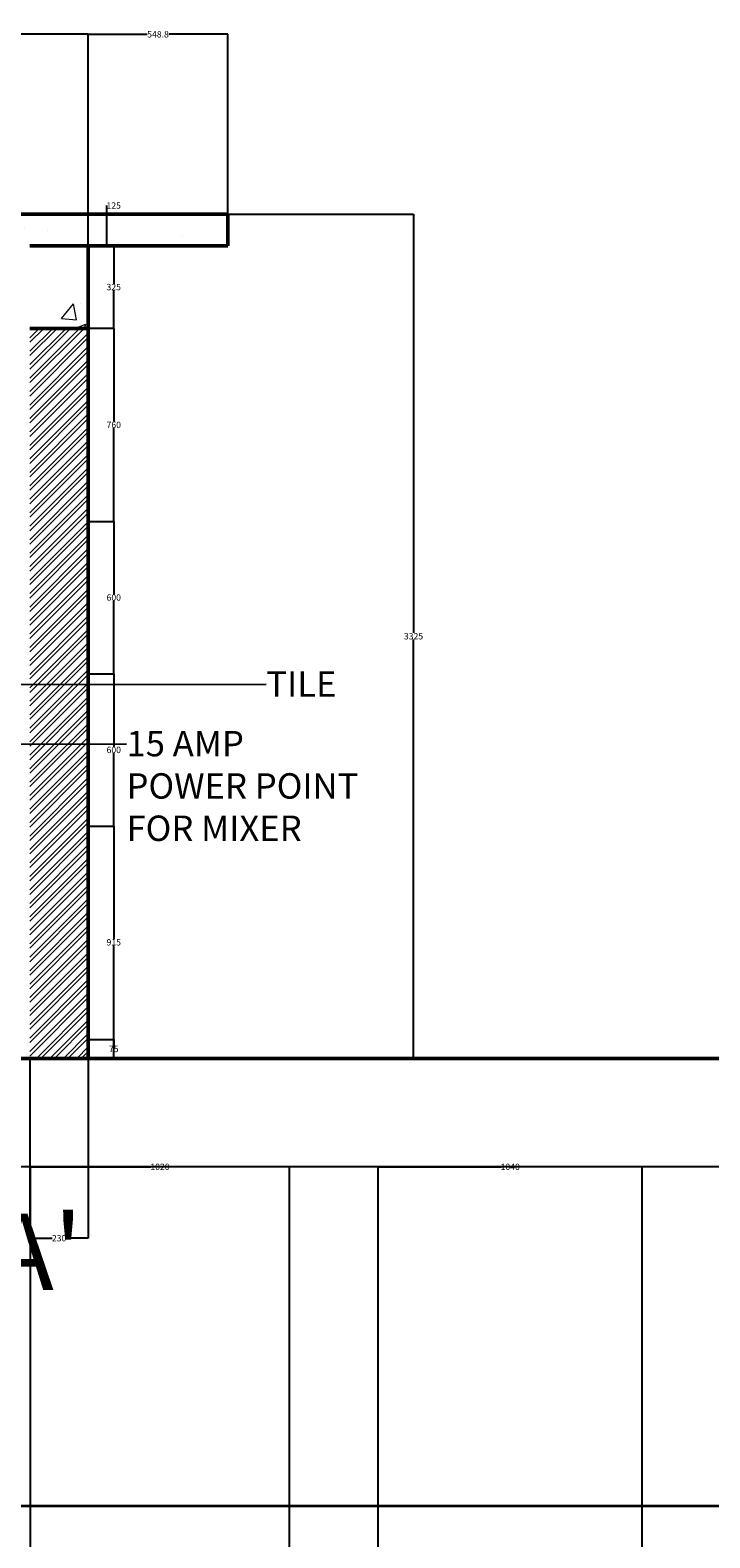
# Model space of a CAD drawing. Units: millimetres. Extents: x 1944 to 29915, y -10550 to 5909.
# Tile 17 of 24: x 16977 to 19652, y -1857 to 4080. Entities that reach past the tile are written whole.
import ezdxf
from ezdxf import colors
from ezdxf.entities.mleader import LeaderData, LeaderLine
from ezdxf.math import Vec2, Vec3

# ---------------------------------------------------------------- set-up
doc = ezdxf.new("R2010")
doc.units = ezdxf.units.MM
doc.header["$MEASUREMENT"] = 0
for name, color, linetype, lineweight in [('A-ANNO-DIMS', 2, 'Continuous', 18), ('A-ANNO-TEXT', 7, 'Continuous', 25), ('A-SECT', 7, 'Continuous', 35), ('A-WALL', 7, 'Continuous', 50), ('A-WALL-PATT', 8, 'Continuous', 18)]:
    doc.layers.add(name, color=color, linetype=linetype, lineweight=lineweight)
doc.styles.get("Standard").update_dxf_attribs({"font": 'arial.ttf'})
doc.dimstyles.get("Standard").update_dxf_attribs({"dimtxt": 25, "dimasz": 0.18, "dimexe": 0.18, "dimexo": 0.0625, "dimgap": 0.09, "dimtad": 0, "dimtih": 1, "dimtoh": 1, "dimdec": 0, "dimzin": 0, "dimdsep": 46, "dimtxsty": 'Standard', "dimcen": 0.09, "dimadec": 0, "dimazin": 0, "dimtfac": 1, "dimtdec": 0, "dimtofl": 0, "dimtmove": 0, "dimatfit": 3, "dimfxl": 1, "dimtolj": 1, "dimtzin": 0, "dimarcsym": 0})

# ---------------------------------------------------------------- blocks, each defined once
blk = doc.blocks.new('*D8')
at = {"layer": 'A-ANNO-DIMS', "color": 0, "lineweight": -2, "transparency": 16777216}
for p, q in [((17205.7, 105.8), (17306.1, 105.8)), ((17305.9, 105.7), (17305.9, 81.1)), ((17205.7, 30.8), (17306.1, 30.8)), ((17305.9, 31), (17305.9, 55.5))]:
    blk.add_line(p, q, dxfattribs=at)
at = {"layer": 'A-ANNO-DIMS', "color": 0, "transparency": 16777216}
for points in [[(17305.9, 105.7), (17305.9, 105.7), (17305.9, 105.8)], [(17305.9, 31), (17305.9, 31), (17305.9, 30.8)]]:
    blk.add_solid(points, dxfattribs=at)
at = {"layer": 'Defpoints', "color": 0, "transparency": 16777216}
for p in [(17205.7, 105.8), (17305.9, 105.8), (17205.7, 30.8)]:
    blk.add_point(p, dxfattribs=at)
at = {"layer": 'A-ANNO-DIMS', "color": 0, "transparency": 16777216, "insert": (17305.9, 68.3), "char_height": 25, "attachment_point": 5}
blk.add_mtext('\\A1;75', dxfattribs=at)
blk = doc.blocks.new('*D9')
at = {"layer": 'A-ANNO-DIMS', "color": 0, "lineweight": -2, "transparency": 16777216}
for p, q in [((17205.7, 945.7), (17306.1, 945.7)), ((17305.9, 945.5), (17305.9, 501)), ((17305.9, 30.8), (17305.9, 475.3)), ((17205.7, 30.7), (17306.1, 30.7))]:
    blk.add_line(p, q, dxfattribs=at)
at = {"layer": 'A-ANNO-DIMS', "color": 0, "transparency": 16777216}
for points in [[(17305.9, 945.5), (17306, 945.5), (17305.9, 945.7)], [(17305.9, 30.8), (17306, 30.8), (17305.9, 30.7)]]:
    blk.add_solid(points, dxfattribs=at)
at = {"layer": 'Defpoints', "color": 0, "transparency": 16777216}
for p in [(17205.7, 945.7), (17305.9, 945.7), (17205.7, 30.7)]:
    blk.add_point(p, dxfattribs=at)
at = {"layer": 'A-ANNO-DIMS', "color": 0, "transparency": 16777216, "insert": (17305.9, 488.2), "char_height": 25, "attachment_point": 5}
blk.add_mtext('\\A1;915', dxfattribs=at)
blk = doc.blocks.new('*D10')
at = {"layer": 'A-ANNO-DIMS', "color": 0, "lineweight": -2, "transparency": 16777216}
for p, q in [((17205.7, 1545.7), (17306.1, 1545.7)), ((17305.9, 1545.5), (17305.9, 1258.5)), ((17305.9, 945.8), (17305.9, 1232.8)), ((17205.7, 945.7), (17306.1, 945.7))]:
    blk.add_line(p, q, dxfattribs=at)
at = {"layer": 'A-ANNO-DIMS', "color": 0, "transparency": 16777216}
for points in [[(17305.9, 1545.5), (17305.9, 1545.5), (17305.9, 1545.7)], [(17305.9, 945.8), (17305.9, 945.8), (17305.9, 945.7)]]:
    blk.add_solid(points, dxfattribs=at)
at = {"layer": 'Defpoints', "color": 0, "transparency": 16777216}
for p in [(17205.7, 1545.7), (17305.9, 1545.7), (17205.7, 945.7)]:
    blk.add_point(p, dxfattribs=at)
at = {"layer": 'A-ANNO-DIMS', "color": 0, "transparency": 16777216, "insert": (17305.9, 1245.7), "char_height": 25, "attachment_point": 5}
blk.add_mtext('\\A1;600', dxfattribs=at)
blk = doc.blocks.new('*D11')
at = {"layer": 'A-ANNO-DIMS', "color": 0, "lineweight": -2, "transparency": 16777216}
for p, q in [((17205.7, 2145.7), (17306.1, 2145.7)), ((17305.9, 2145.5), (17305.9, 1858.5)), ((17305.9, 1545.8), (17305.9, 1832.8)), ((17205.7, 1545.7), (17306.1, 1545.7))]:
    blk.add_line(p, q, dxfattribs=at)
at = {"layer": 'A-ANNO-DIMS', "color": 0, "transparency": 16777216}
for points in [[(17305.9, 2145.5), (17305.9, 2145.5), (17305.9, 2145.7)], [(17305.9, 1545.8), (17305.9, 1545.8), (17305.9, 1545.7)]]:
    blk.add_solid(points, dxfattribs=at)
at = {"layer": 'Defpoints', "color": 0, "transparency": 16777216}
for p in [(17205.7, 2145.7), (17305.9, 2145.7), (17205.7, 1545.7)]:
    blk.add_point(p, dxfattribs=at)
at = {"layer": 'A-ANNO-DIMS', "color": 0, "transparency": 16777216, "insert": (17305.9, 1845.7), "char_height": 25, "attachment_point": 5}
blk.add_mtext('\\A1;600', dxfattribs=at)
blk = doc.blocks.new('*D12')
at = {"layer": 'A-ANNO-DIMS', "color": 0, "lineweight": -2, "transparency": 16777216}
for p, q in [((17205.7, 2905.7), (17306.1, 2905.7)), ((17305.9, 2905.5), (17305.9, 2538.5)), ((17305.9, 2145.8), (17305.9, 2512.8)), ((17205.7, 2145.7), (17306.1, 2145.7))]:
    blk.add_line(p, q, dxfattribs=at)
at = {"layer": 'A-ANNO-DIMS', "color": 0, "transparency": 16777216}
for points in [[(17305.9, 2905.5), (17306, 2905.5), (17305.9, 2905.7)], [(17305.9, 2145.8), (17306, 2145.8), (17305.9, 2145.7)]]:
    blk.add_solid(points, dxfattribs=at)
at = {"layer": 'Defpoints', "color": 0, "transparency": 16777216}
for p in [(17205.7, 2905.7), (17305.9, 2905.7), (17205.7, 2145.7)]:
    blk.add_point(p, dxfattribs=at)
at = {"layer": 'A-ANNO-DIMS', "color": 0, "transparency": 16777216, "insert": (17305.9, 2525.7), "char_height": 25, "attachment_point": 5}
blk.add_mtext('\\A1;760', dxfattribs=at)
blk = doc.blocks.new('*D13')
at = {"layer": 'A-ANNO-DIMS', "color": 0, "lineweight": -2, "transparency": 16777216}
for p, q in [((17205.7, 3230.5), (17305.7, 3230.5)), ((17305.6, 3230.3), (17305.6, 3080.9)), ((17305.6, 2905.8), (17305.6, 3055.2)), ((17205.7, 2905.7), (17305.7, 2905.7))]:
    blk.add_line(p, q, dxfattribs=at)
at = {"layer": 'A-ANNO-DIMS', "color": 0, "transparency": 16777216}
for points in [[(17305.5, 3230.3), (17305.6, 3230.3), (17305.6, 3230.5)], [(17305.5, 2905.8), (17305.6, 2905.8), (17305.6, 2905.7)]]:
    blk.add_solid(points, dxfattribs=at)
at = {"layer": 'Defpoints', "color": 0, "transparency": 16777216}
for p in [(17205.7, 3230.5), (17305.6, 3230.5), (17205.7, 2905.7)]:
    blk.add_point(p, dxfattribs=at)
at = {"layer": 'A-ANNO-DIMS', "color": 0, "transparency": 16777216, "insert": (17305.6, 3068.1), "char_height": 25, "attachment_point": 5}
blk.add_mtext('\\A1;325', dxfattribs=at)
blk = doc.blocks.new('*D14')
at = {"layer": 'A-ANNO-DIMS', "color": 0, "lineweight": -2, "transparency": 16777216}
for p, q in [((17278.8, 3355.7), (17278.8, 3389.1)), ((17278.8, 3389.1), (17278.9, 3389.1)), ((17305.7, 3355.7), (17278.6, 3355.7)), ((17278.8, 3230.8), (17278.8, 3355.5)), ((17305.7, 3230.7), (17278.6, 3230.7))]:
    blk.add_line(p, q, dxfattribs=at)
at = {"layer": 'A-ANNO-DIMS', "color": 0, "transparency": 16777216}
for points in [[(17278.7, 3355.5), (17278.8, 3355.5), (17278.8, 3355.7)], [(17278.7, 3230.8), (17278.8, 3230.8), (17278.8, 3230.7)]]:
    blk.add_solid(points, dxfattribs=at)
at = {"layer": 'Defpoints', "color": 0, "transparency": 16777216}
for p in [(17278.8, 3355.7), (17305.7, 3355.7), (17305.7, 3230.7)]:
    blk.add_point(p, dxfattribs=at)
at = {"layer": 'A-ANNO-DIMS', "color": 0, "transparency": 16777216, "insert": (17305.6, 3389.1), "char_height": 25, "attachment_point": 5}
blk.add_mtext('\\A1;125', dxfattribs=at)
blk = doc.blocks.new('*D22')
at = {"layer": 'A-ANNO-DIMS', "color": 0, "lineweight": -2, "transparency": 16777216}
for p, q in [((17754.5, 3355.7), (18486.1, 3355.7)), ((18485.9, 3355.5), (18485.9, 1706.1)), ((18485.9, 31), (18485.9, 1680.4)), ((17306, 30.8), (18486.1, 30.8))]:
    blk.add_line(p, q, dxfattribs=at)
at = {"layer": 'A-ANNO-DIMS', "color": 0, "transparency": 16777216}
for points in [[(18485.9, 3355.5), (18485.9, 3355.5), (18485.9, 3355.7)], [(18485.9, 31), (18485.9, 31), (18485.9, 30.8)]]:
    blk.add_solid(points, dxfattribs=at)
at = {"layer": 'Defpoints', "color": 0, "transparency": 16777216}
for p in [(17754.5, 3355.7), (17305.9, 30.8), (18485.9, 30.8)]:
    blk.add_point(p, dxfattribs=at)
at = {"layer": 'A-ANNO-DIMS', "color": 0, "transparency": 16777216, "insert": (18485.9, 1693.2), "char_height": 25, "attachment_point": 5}
blk.add_mtext('\\A1;3325', dxfattribs=at)
blk = doc.blocks.new('*D61')
at = {"layer": 'A-ANNO-DIMS', "color": 0, "lineweight": -2, "transparency": 16777216}
for p, q in [((12776.5, 3230.7), (12776.5, 4063.5)), ((12776.7, 4063.3), (14953.2, 4063.3)), ((17205.5, 4063.3), (15029.1, 4063.3)), ((17205.7, 3230.7), (17205.7, 4063.5))]:
    blk.add_line(p, q, dxfattribs=at)
at = {"layer": 'A-ANNO-DIMS', "color": 0, "transparency": 16777216}
for points in [[(12776.7, 4063.4), (12776.7, 4063.3), (12776.5, 4063.3)], [(17205.5, 4063.4), (17205.5, 4063.3), (17205.7, 4063.3)]]:
    blk.add_solid(points, dxfattribs=at)
at = {"layer": 'Defpoints', "color": 0, "transparency": 16777216}
for p in [(17205.7, 4063.3), (12776.5, 3230.7), (17205.7, 3230.7)]:
    blk.add_point(p, dxfattribs=at)
at = {"layer": 'A-ANNO-DIMS', "color": 0, "transparency": 16777216, "insert": (14991.1, 4063.3), "char_height": 25, "attachment_point": 5}
blk.add_mtext('\\A1;4429', dxfattribs=at)
blk = doc.blocks.new('*D62')
at = {"layer": 'A-ANNO-DIMS', "color": 0, "lineweight": -2, "transparency": 16777216}
for p, q in [((17205.7, 3230.7), (17205.7, 4063.5)), ((17205.8, 4063.3), (17437.8, 4063.3)), ((17754.3, 4063.3), (17522.4, 4063.3)), ((17754.5, 3230.5), (17754.5, 4063.5))]:
    blk.add_line(p, q, dxfattribs=at)
at = {"layer": 'A-ANNO-DIMS', "color": 0, "transparency": 16777216}
for points in [[(17205.8, 4063.4), (17205.8, 4063.3), (17205.7, 4063.3)], [(17754.3, 4063.4), (17754.3, 4063.3), (17754.5, 4063.3)]]:
    blk.add_solid(points, dxfattribs=at)
at = {"layer": 'Defpoints', "color": 0, "transparency": 16777216}
for p in [(17754.5, 4063.3), (17205.7, 3230.7), (17754.5, 3230.5)]:
    blk.add_point(p, dxfattribs=at)
at = {"layer": 'A-ANNO-DIMS', "color": 0, "transparency": 16777216, "insert": (17480.1, 4063.3), "char_height": 25, "attachment_point": 5}
blk.add_mtext('\\A1;548.8', dxfattribs=at)
blk = doc.blocks.new('*D71')
at = {"layer": 'A-ANNO-DIMS', "color": 0, "lineweight": -2, "transparency": 16777216}
for p, q in [((16975.7, 30.8), (16975.7, -677)), ((17205.7, 30.8), (17205.7, -677)), ((16975.8, -676.8), (17062.8, -676.8)), ((17205.5, -676.8), (17118.5, -676.8))]:
    blk.add_line(p, q, dxfattribs=at)
at = {"layer": 'A-ANNO-DIMS', "color": 0, "transparency": 16777216}
for points in [[(16975.8, -676.8), (16975.8, -676.9), (16975.7, -676.8)], [(17205.5, -676.8), (17205.5, -676.9), (17205.7, -676.8)]]:
    blk.add_solid(points, dxfattribs=at)
at = {"layer": 'Defpoints', "color": 0, "transparency": 16777216}
for p in [(16975.7, 30.8), (17205.7, 30.8), (17205.7, -676.8)]:
    blk.add_point(p, dxfattribs=at)
at = {"layer": 'A-ANNO-DIMS', "color": 0, "transparency": 16777216, "insert": (17090.7, -676.8), "char_height": 25, "attachment_point": 5}
blk.add_mtext('\\A1;230', dxfattribs=at)
blk = doc.blocks.new('*D85')
at = {"layer": 'A-ANNO-DIMS', "color": 0, "lineweight": -2, "transparency": 16777216}
for p, q in [((6418.3, -1730.7), (6418.3, -395.6)), ((6418.5, -395.8), (15860.3, -395.8)), ((25389.1, -395.8), (15947.3, -395.8)), ((25389.3, -1846.5), (25389.3, -395.6))]:
    blk.add_line(p, q, dxfattribs=at)
at = {"layer": 'A-ANNO-DIMS', "color": 0, "transparency": 16777216}
for points in [[(6418.5, -395.7), (6418.5, -395.8), (6418.3, -395.8)], [(25389.1, -395.7), (25389.1, -395.8), (25389.3, -395.8)]]:
    blk.add_solid(points, dxfattribs=at)
at = {"layer": 'Defpoints', "color": 0, "transparency": 16777216}
for p in [(25389.3, -395.8), (6418.3, -1730.8), (25389.3, -1846.5)]:
    blk.add_point(p, dxfattribs=at)
at = {"layer": 'A-ANNO-DIMS', "color": 0, "transparency": 16777216, "insert": (15903.8, -395.8), "char_height": 25, "attachment_point": 5}
blk.add_mtext('\\A1;18971', dxfattribs=at)
blk = doc.blocks.new('*D94')
at = {"layer": 'A-ANNO-DIMS', "color": 0, "lineweight": -2, "transparency": 16777216}
for p, q in [((16977.8, -3070.7), (16977.8, -395.6)), ((16978, -395.8), (17451.6, -395.8)), ((17997.6, -395.8), (17524, -395.8)), ((17997.8, -3070.7), (17997.8, -395.6))]:
    blk.add_line(p, q, dxfattribs=at)
at = {"layer": 'A-ANNO-DIMS', "color": 0, "transparency": 16777216}
for points in [[(16978, -395.7), (16978, -395.8), (16977.8, -395.8)], [(17997.6, -395.7), (17997.6, -395.8), (17997.8, -395.8)]]:
    blk.add_solid(points, dxfattribs=at)
at = {"layer": 'Defpoints', "color": 0, "transparency": 16777216}
for p in [(17997.8, -395.8), (16977.8, -3070.8), (17997.8, -3070.8)]:
    blk.add_point(p, dxfattribs=at)
at = {"layer": 'A-ANNO-DIMS', "color": 0, "transparency": 16777216, "insert": (17487.8, -395.8), "char_height": 25, "attachment_point": 5}
blk.add_mtext('\\A1;1020', dxfattribs=at)
blk = doc.blocks.new('*D95')
at = {"layer": 'A-ANNO-DIMS', "color": 0, "lineweight": -2, "transparency": 16777216}
for p, q in [((18346.6, -3070.7), (18346.6, -395.6)), ((18346.8, -395.8), (18830.4, -395.8)), ((19386.5, -395.8), (18902.8, -395.8)), ((19386.6, -3070.7), (19386.6, -395.6))]:
    blk.add_line(p, q, dxfattribs=at)
at = {"layer": 'A-ANNO-DIMS', "color": 0, "transparency": 16777216}
for points in [[(18346.8, -395.7), (18346.8, -395.8), (18346.6, -395.8)], [(19386.5, -395.7), (19386.5, -395.8), (19386.6, -395.8)]]:
    blk.add_solid(points, dxfattribs=at)
at = {"layer": 'Defpoints', "color": 0, "transparency": 16777216}
for p in [(19386.6, -395.8), (18346.6, -3070.8), (19386.6, -3070.8)]:
    blk.add_point(p, dxfattribs=at)
at = {"layer": 'A-ANNO-DIMS', "color": 0, "transparency": 16777216, "insert": (18866.6, -395.8), "char_height": 25, "attachment_point": 5}
blk.add_mtext('\\A1;1040', dxfattribs=at)

msp = doc.modelspace()

# ---------------------------------------------------------------- hatches: boundary and pattern name
at = {"layer": 'A-WALL-PATT'}
h = msp.add_hatch(dxfattribs=at)
h.set_pattern_fill('AR-CONC', color=256, scale=100)
h.paths.add_polyline_path([(17754.476, 3355.657), (12150.994, 3355.657), (12150.994, 3230.657), (16975.67, 3230.657), (16975.67, 2907.477), (17205.67, 2907.477), (17205.67, 3230.657), (17754.476, 3230.657)])
h = msp.add_hatch(dxfattribs=at)
h.set_pattern_fill('ANSI32', color=256, scale=100)
h.paths.add_polyline_path([(17205.67, 2905.657), (16975.67, 2905.657), (16975.67, 30.837), (17205.67, 30.837)])

# ---------------------------------------------------------------- linework, layer by layer
at = {"layer": 'A-SECT'}
msp.add_line((16516.552, -1730.752), (20985.45, -1730.752), dxfattribs=at)
at = {"layer": 'A-WALL'}
for p, q in [((12150.994, 3355.657), (17754.476, 3355.657)), ((17754.476, 3355.657), (17754.476, 3230.477)), ((17754.476, 3230.477), (16975.67, 3230.477)), ((17205.67, 30.837), (17205.67, 3230.657)), ((17205.67, 2905.657), (16975.67, 2905.657)), ((24504.139, 30.837), (12776.548, 30.837))]:
    msp.add_line(p, q, dxfattribs=at)

# ---------------------------------------------------------------- texts
at = {"layer": 'A-ANNO-TEXT'}
msp.add_text("SECTION - AT 'A'", height=300, dxfattribs=at).set_placement((14085.235, -880.236))

# ---------------------------------------------------------------- dimensions: what is measured, and where the dimension line sits
at = {"layer": 'A-ANNO-DIMS'}
for base, p1, p2, override, picture, middle in [((17205.67, 4063.337), (12776.548, 3230.657), (17205.67, 3230.657), {"dimdec": 0, "dimlfac": 1, "dimrnd": 0, "dimzin": 0, "dimdsep": 46, "dimlunit": 2}, '*D61', (14991.109, 4063.337)), ((17754.476, 4063.337), (17205.67, 3230.657), (17754.476, 3230.477), {"dimdec": 1, "dimlfac": 1, "dimrnd": 0, "dimzin": 0, "dimdsep": 46, "dimlunit": 2}, '*D62', (17480.073, 4063.337)), ((17205.67, -676.843), (16975.67, 30.837), (17205.67, 30.837), {"dimdec": 0, "dimlfac": 1, "dimrnd": 0, "dimzin": 0, "dimdsep": 46, "dimlunit": 2}, '*D71', (17090.67, -676.843)), ((25389.297, -395.752), (6418.315, -1730.752), (25389.297, -1846.542), {"dimdec": 0, "dimlfac": 1, "dimrnd": 0, "dimzin": 0, "dimdsep": 46, "dimlunit": 2}, '*D85', (15903.806, -395.752)), ((17997.828, -395.752), (16977.828, -3070.752), (17997.828, -3070.752), {"dimdec": 0, "dimlfac": 1, "dimrnd": 0, "dimzin": 0, "dimdsep": 46, "dimlunit": 2}, '*D94', (17487.828, -395.752)), ((19386.639, -395.752), (18346.639, -3070.752), (19386.639, -3070.752), {"dimdec": 0, "dimlfac": 1, "dimrnd": 0, "dimzin": 0, "dimdsep": 46, "dimlunit": 2}, '*D95', (18866.639, -395.752))]:
    dim = msp.add_linear_dim(base=base, p1=p1, p2=p2, dimstyle='Standard', override=override, dxfattribs=at)
    dim.commit()
    dim.dimension.update_dxf_attribs({"geometry": picture, "text_midpoint": middle})
dim = msp.add_linear_dim(base=(17278.753, 3355.657), p1=(17305.738, 3230.657), p2=(17305.738, 3355.657), angle=90, dimstyle='Standard', override={"dimclrd": 0, "dimclre": 0, "dimclrt": 0}, dxfattribs=at)
dim.commit()
dim.dimension.update_dxf_attribs({"geometry": '*D14', "text_midpoint": (17305.558, 3389.084), "dimtype": 160})
for base, p1, p2, picture, middle in [((18485.912, 30.837), (17754.476, 3355.657), (17305.908, 30.837), '*D22', (18485.912, 1693.247)), ((17305.558, 3230.477), (17205.67, 2905.657), (17205.67, 3230.477), '*D13', (17305.558, 3068.067)), ((17305.938, 2905.657), (17205.67, 2145.657), (17205.67, 2905.657), '*D12', (17305.938, 2525.657)), ((17305.908, 2145.657), (17205.67, 1545.657), (17205.67, 2145.657), '*D11', (17305.908, 1845.657)), ((17305.908, 1545.657), (17205.67, 945.657), (17205.67, 1545.657), '*D10', (17305.908, 1245.657)), ((17305.938, 945.657), (17205.67, 30.657), (17205.67, 945.657), '*D9', (17305.938, 488.157)), ((17305.908, 105.837), (17205.67, 30.837), (17205.67, 105.837), '*D8', (17305.908, 68.337))]:
    dim = msp.add_linear_dim(base=base, p1=p1, p2=p2, angle=90, dimstyle='Standard', override={"dimclrd": 0, "dimclre": 0, "dimclrt": 0}, dxfattribs=at)
    dim.commit()
    dim.dimension.update_dxf_attribs({"geometry": picture, "text_midpoint": middle})

# ---------------------------------------------------------------- leaders
at = {"layer": 'A-ANNO-TEXT'}
ml = msp.add_multileader_mtext('Standard', dxfattribs=at)
ml.set_content('TILE ', color=256)
ml.set_leader_properties()
ml.build(insert=Vec2(0, 0))
ml.multileader.update_dxf_attribs({"dogleg_length": 0.36, "arrow_head_size": 100})
ctx = ml.context
ctx.base_point, ctx.char_height, ctx.arrow_head_size, ctx.landing_gap_size, ctx.plane_origin = Vec3(17906.299, 1505.142), 100, 100, 0.09, Vec3(17905.939, 1505.142)
notes = []
notes.append((ctx, [(0, (1, 1, 0), (17905.939, 1505.142), (1, 0), 0.36, [(0, [(16303.171, 1501.973)], 0, [])])]))
ctx.mtext.insert, ctx.mtext.flow_direction = Vec3(17906.389, 1555.142), 5
ml = msp.add_multileader_mtext('Standard', dxfattribs=at)
ml.set_content('15 AMP\\PPOWER POINT \\PFOR MIXER ', color=256)
ml.set_leader_properties()
ml.build(insert=Vec2(0, 0))
ml.multileader.update_dxf_attribs({"dogleg_length": 0.36, "arrow_head_size": 100})
ctx = ml.context
ctx.base_point, ctx.char_height, ctx.arrow_head_size, ctx.landing_gap_size, ctx.plane_origin = Vec3(17355.956, 1269.694), 100, 100, 0.09, Vec3(17355.596, 1269.694)
notes.append((ctx, [(0, (1, 1, 0), (17355.596, 1269.694), (1, 0), 0.36, [(0, [(15752.828, 1266.525)], 0, [])])]))
ctx.mtext.insert, ctx.mtext.flow_direction = Vec3(17356.046, 1320.547), 5
for ctx, leaders in notes:
    for number, flags, end, landing, length, lines in leaders:
        leader = LeaderData()
        leader.index, (leader.has_last_leader_line, leader.has_dogleg_vector, leader.attachment_direction) = number, flags
        leader.last_leader_point, leader.dogleg_vector, leader.dogleg_length = Vec3(end), Vec3(landing), length
        for number, points, colour, breaks in lines:
            line = LeaderLine()
            line.index, line.vertices, line.color, line.breaks = number, Vec3.list(points), colors.encode_raw_color(colour), breaks
            leader.lines.append(line)
        ctx.leaders.append(leader)

doc.saveas('drawing.dxf')
